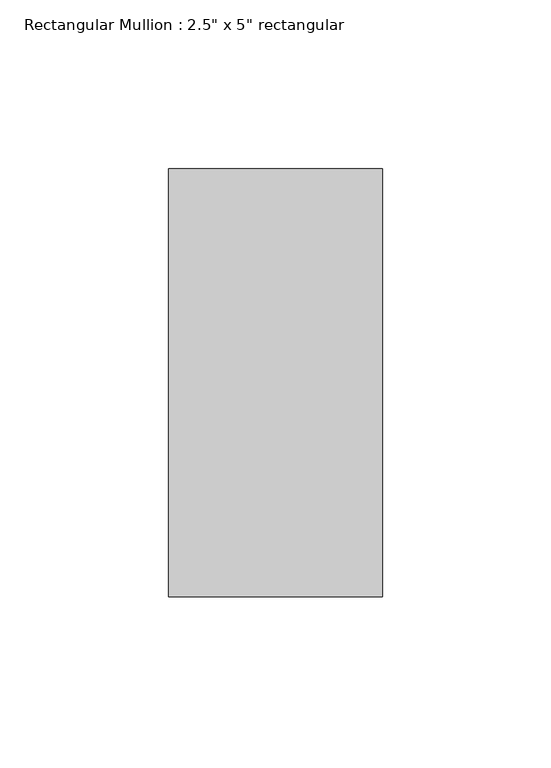
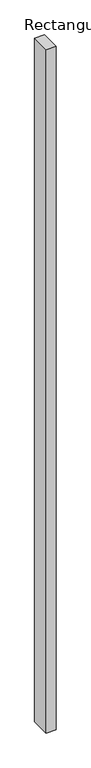
"""IFC4 building model written with IfcOpenShell, lengths in millimetres: member geometry."""

from ifc_helpers import new_model, si_unit, frame, origin, place, context, project, spatial, polyline, outline, extrude, source, transform, mapped, element, save


def member_43964152(model_context):
    return source(origin(), model_context, "Body", "SweptSolid", [
        extrude(outline(polyline([(0.0, 63.5), (0.0, -63.5), (-63.5, -63.5), (-63.5, 63.5), (0.0, 63.5)])), frame((0.0, 0.0, -4642.1208035), z_axis=(0.0, 0.0, 1.0), x_axis=(1.0, 0.0, 0.0)), (0.0, 0.0, 1.0), 4642.1208035),
    ])


if __name__ == "__main__":
    model = new_model("IFC4")
    model_context = context("Model", 3, world=origin())
    ifc_project = project(units=[si_unit("LENGTHUNIT", "METRE", prefix="MILLI")], contexts=[model_context])
    site = spatial("IfcSite", under=ifc_project)
    building = spatial("IfcBuilding", under=site)
    placement = place(None, origin())
    member_shape = member_43964152(model_context)
    element("IfcMember", 1, ObjectType="Rectangular Mullion : 2.5\" x 5\" rectangular", at=placement, inside=building, context=model_context, shape_type="MappedRepresentation", body=[
        mapped(member_shape, transform((0.0, 0.0, 0.0), x_axis=(1.0, 0.0, 0.0), y_axis=(0.0, 1.0, 0.0), z_axis=(0.0, 0.0, 1.0))),
    ])
    save(model, "model.ifc")

# Revit data of these elements
# Type "Rectangular Mullion : 2.5\" x 5\" rectangular"
#   built-in parameter 1007304 = 0.416667 (stored number, unit not read)
#   built-in parameter 1007301 = 0.104167 (stored number, unit not read)
#   built-in parameter 1007300 = 0.104167 (stored number, unit not read)
# Element 1 (IfcMember, "Rectangular Mullion : 2.5\" x 5\" rectangular")
#   Materials on its faces: "Aluminum"
# Materials
#   "Aluminum": class "Metal", colour RGB 247 247 247, transparency 0, Description = "Aluminum 6061", Cost = 0
